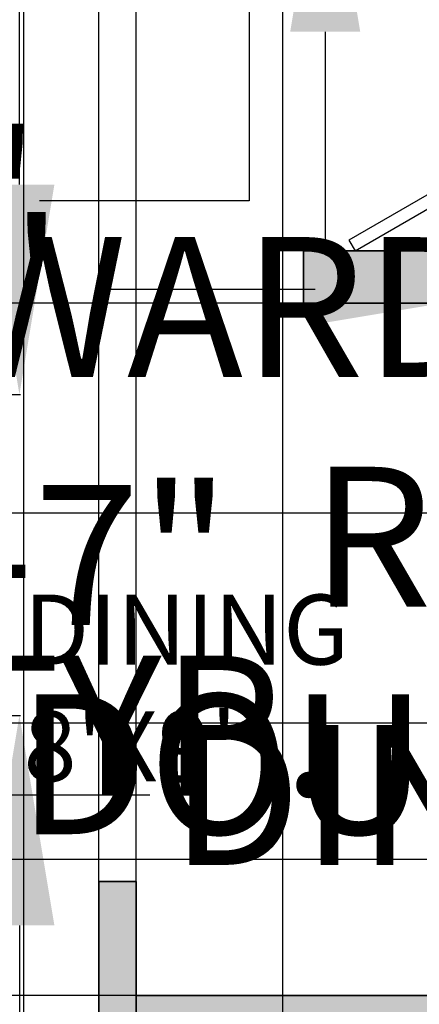
# Model space of a CAD drawing. Units: inches. Extents: x 2838 to 4029, y 1041 to 1915.
# Tile 8 of 16: x 3441 to 3510, y 1377 to 1546. Entities that reach past the tile are written whole.
import ezdxf

# ---------------------------------------------------------------- set-up
doc = ezdxf.new("R2010")
doc.units = ezdxf.units.IN
doc.header["$MEASUREMENT"] = 0
for name, color, linetype, lineweight in [('A-ANNO-DIMS', 2, 'Continuous', 18), ('A-AREA-IDEN', 7, 'Continuous', 18), ('A-DOOR', 3, 'Continuous', 25), ('A-WALL', 7, 'Continuous', 35), ('A-WALL-PATT', 252, 'Continuous', 13)]:
    doc.layers.add(name, color=color, linetype=linetype, lineweight=lineweight)
doc.styles.get("Standard").update_dxf_attribs({"font": 'arial.ttf'})
doc.dimstyles.get("Standard").update_dxf_attribs({"dimtxt": 24, "dimasz": 36, "dimexe": 0.18, "dimexo": 0.0625, "dimgap": 0.09, "dimtad": 0, "dimtih": 1, "dimtoh": 1, "dimdec": 0, "dimzin": 0, "dimdsep": 46, "dimlunit": 3, "dimtxsty": 'Standard', "dimcen": 0.09, "dimadec": 0, "dimazin": 0, "dimtfac": 1, "dimtdec": 0, "dimtofl": 0, "dimtmove": 0, "dimatfit": 3, "dimfxl": 1, "dimtolj": 1, "dimtzin": 0, "dimarcsym": 0})

# ---------------------------------------------------------------- blocks, each defined once
blk = doc.blocks.new('*U3')
for p, q in [((-40, 0), (-40, 6)), ((0, 0), (0, 6))]:
    blk.add_line(p, q)
blk.add_lwpolyline([(0, 0), (-20, -34.64), (-21.52, -33.77), (-1.52, 0.88)], close=True)
blk.add_arc((0, 0), 40, 180, 240)
blk = doc.blocks.new('*D26')
at = {"layer": 'A-ANNO-DIMS', "color": 0, "lineweight": -2, "transparency": 16777216}
for p, q in [((3267.73, 1432.1), (3267.73, 1424.79)), ((3276.73, 1432.1), (3276.73, 1424.79)), ((3231.73, 1424.97), (3195.73, 1424.97)), ((3312.73, 1424.97), (3348.73, 1424.97))]:
    blk.add_line(p, q, dxfattribs=at)
at = {"layer": 'A-ANNO-DIMS', "color": 0, "transparency": 16777216}
for points in [[(3231.73, 1430.97), (3231.73, 1418.97), (3267.73, 1424.97)], [(3312.73, 1430.97), (3312.73, 1418.97), (3276.73, 1424.97)]]:
    blk.add_solid(points, dxfattribs=at)
at = {"layer": 'Defpoints', "color": 0, "transparency": 16777216}
for p in [(3267.73, 1432.17), (3276.73, 1432.17), (3276.73, 1424.97)]:
    blk.add_point(p, dxfattribs=at)
at = {"layer": 'A-ANNO-DIMS', "color": 0, "transparency": 16777216, "insert": (3421.97, 1424.97), "char_height": 24, "attachment_point": 5}
blk.add_mtext('\\A1;0\'-9" TYP.', dxfattribs=at)
blk = doc.blocks.new('*D33')
at = {"layer": 'A-ANNO-DIMS', "color": 0, "lineweight": -2, "transparency": 16777216}
for p, q in [((3601.73, 1469.45), (3601.73, 1505.45)), ((3603.48, 1433.45), (3601.55, 1433.45)), ((3603.48, 1421.37), (3601.55, 1421.37)), ((3601.73, 1385.37), (3601.73, 1349.37)), ((3601.73, 1349.37), (3565.73, 1349.37))]:
    blk.add_line(p, q, dxfattribs=at)
at = {"layer": 'A-ANNO-DIMS', "color": 0, "transparency": 16777216}
for points in [[(3595.73, 1469.45), (3607.73, 1469.45), (3601.73, 1433.45)], [(3595.73, 1385.37), (3607.73, 1385.37), (3601.73, 1421.37)]]:
    blk.add_solid(points, dxfattribs=at)
at = {"layer": 'Defpoints', "color": 0, "transparency": 16777216}
for p in [(3603.54, 1433.45), (3601.73, 1421.37), (3603.54, 1421.37)]:
    blk.add_point(p, dxfattribs=at)
at = {"layer": 'A-ANNO-DIMS', "color": 0, "transparency": 16777216, "insert": (3496.18, 1349.37), "char_height": 24, "attachment_point": 5}
blk.add_mtext('\\A1;TAP 1\'-0"', dxfattribs=at)
blk = doc.blocks.new('*D35')
at = {"layer": 'A-ANNO-DIMS', "color": 0, "lineweight": -2, "transparency": 16777216}
for p, q in [((3480.45, 1632.93), (3480.45, 1668.93)), ((3481.89, 1596.93), (3480.27, 1596.93)), ((3481.89, 1586.93), (3480.27, 1586.93)), ((3480.45, 1550.93), (3480.45, 1514.93)), ((3480.45, 1514.93), (3444.45, 1514.93))]:
    blk.add_line(p, q, dxfattribs=at)
at = {"layer": 'A-ANNO-DIMS', "color": 0, "transparency": 16777216}
for points in [[(3474.45, 1632.93), (3486.45, 1632.93), (3480.45, 1596.93)], [(3474.45, 1550.93), (3486.45, 1550.93), (3480.45, 1586.93)]]:
    blk.add_solid(points, dxfattribs=at)
at = {"layer": 'Defpoints', "color": 0, "transparency": 16777216}
for p in [(3481.95, 1596.93), (3480.45, 1586.93), (3481.95, 1586.93)]:
    blk.add_point(p, dxfattribs=at)
at = {"layer": 'A-ANNO-DIMS', "color": 0, "transparency": 16777216, "insert": (3365.58, 1514.93), "char_height": 24, "attachment_point": 5}
blk.add_mtext('\\A1;TAP 0\'-10"', dxfattribs=at)
blk = doc.blocks.new('*D41')
at = {"layer": 'A-ANNO-DIMS', "color": 0, "lineweight": -2, "transparency": 16777216}
for p, q in [((3284.24, 1506.2), (3284.24, 1496.56)), ((3347.73, 1506.2), (3347.73, 1496.56)), ((3248.24, 1496.74), (3212.24, 1496.74)), ((3383.73, 1496.74), (3419.73, 1496.74))]:
    blk.add_line(p, q, dxfattribs=at)
at = {"layer": 'A-ANNO-DIMS', "color": 0, "transparency": 16777216}
for points in [[(3248.24, 1502.74), (3248.24, 1490.74), (3284.24, 1496.74)], [(3383.73, 1502.74), (3383.73, 1490.74), (3347.73, 1496.74)]]:
    blk.add_solid(points, dxfattribs=at)
at = {"layer": 'Defpoints', "color": 0, "transparency": 16777216}
for p in [(3284.24, 1506.26), (3347.73, 1506.26), (3347.73, 1496.74)]:
    blk.add_point(p, dxfattribs=at)
at = {"layer": 'A-ANNO-DIMS', "color": 0, "transparency": 16777216, "insert": (3624.81, 1496.74), "char_height": 24, "attachment_point": 5}
blk.add_mtext('\\A1;WARDROBE 5\'-3 1/2" TYP.', dxfattribs=at)
blk = doc.blocks.new('*D47')
at = {"layer": 'A-ANNO-DIMS', "color": 0, "lineweight": -2, "transparency": 16777216}
for p, q in [((3493.47, 1640.5), (3493.47, 1676.5)), ((3493.47, 1676.5), (3529.47, 1676.5)), ((3489.85, 1604.5), (3493.65, 1604.5)), ((3489.85, 1579.95), (3493.65, 1579.95)), ((3493.47, 1543.95), (3493.47, 1507.95))]:
    blk.add_line(p, q, dxfattribs=at)
at = {"layer": 'A-ANNO-DIMS', "color": 0, "transparency": 16777216}
for points in [[(3487.47, 1640.5), (3499.47, 1640.5), (3493.47, 1604.5)], [(3487.47, 1543.95), (3499.47, 1543.95), (3493.47, 1579.95)]]:
    blk.add_solid(points, dxfattribs=at)
at = {"layer": 'Defpoints', "color": 0, "transparency": 16777216}
for p in [(3489.78, 1604.5), (3493.47, 1604.5), (3489.78, 1579.95)]:
    blk.add_point(p, dxfattribs=at)
at = {"layer": 'A-ANNO-DIMS', "color": 0, "transparency": 16777216, "insert": (3643.85, 1676.5), "char_height": 24, "attachment_point": 5}
blk.add_mtext('\\A1;BASIN 2\'-0 1/2"', dxfattribs=at)
blk = doc.blocks.new('*D49')
at = {"layer": 'A-ANNO-DIMS', "color": 0, "lineweight": -2, "transparency": 16777216}
for p, q in [((3336.37, 1426.68), (3336.37, 1412.92)), ((3427.37, 1426.68), (3427.37, 1412.92)), ((3372.37, 1413.1), (3391.37, 1413.1)), ((3427.37, 1413.1), (3463.37, 1413.1))]:
    blk.add_line(p, q, dxfattribs=at)
at = {"layer": 'A-ANNO-DIMS', "color": 0, "transparency": 16777216}
for points in [[(3372.37, 1419.1), (3372.37, 1407.1), (3336.37, 1413.1)], [(3391.37, 1419.1), (3391.37, 1407.1), (3427.37, 1413.1)]]:
    blk.add_solid(points, dxfattribs=at)
at = {"layer": 'Defpoints', "color": 0, "transparency": 16777216}
for p in [(3336.37, 1426.75), (3427.37, 1426.75), (3427.37, 1413.1)]:
    blk.add_point(p, dxfattribs=at)
at = {"layer": 'A-ANNO-DIMS', "color": 0, "transparency": 16777216, "insert": (3595.36, 1413.1), "char_height": 24, "attachment_point": 5}
blk.add_mtext('\\A1;DINING SET 7\'-7"', dxfattribs=at)
blk = doc.blocks.new('*D50')
at = {"layer": 'A-ANNO-DIMS', "color": 0, "lineweight": -2, "transparency": 16777216}
for p, q in [((3441.02, 1517.75), (3441.02, 1553.75)), ((3427.44, 1481.75), (3441.2, 1481.75)), ((3427.44, 1426.75), (3441.2, 1426.75)), ((3441.02, 1390.75), (3441.02, 1354.75))]:
    blk.add_line(p, q, dxfattribs=at)
at = {"layer": 'A-ANNO-DIMS', "color": 0, "transparency": 16777216}
for points in [[(3435.02, 1517.75), (3447.02, 1517.75), (3441.02, 1481.75)], [(3435.02, 1390.75), (3447.02, 1390.75), (3441.02, 1426.75)]]:
    blk.add_solid(points, dxfattribs=at)
at = {"layer": 'Defpoints', "color": 0, "transparency": 16777216}
for p in [(3427.37, 1481.75), (3441.02, 1481.75), (3427.37, 1426.75)]:
    blk.add_point(p, dxfattribs=at)
at = {"layer": 'A-ANNO-DIMS', "color": 0, "transparency": 16777216, "insert": (3441.02, 1454.25), "char_height": 24, "attachment_point": 5}
blk.add_mtext('\\A1;4\'-7"', dxfattribs=at)
blk = doc.blocks.new('*D53')
at = {"layer": 'A-ANNO-DIMS', "color": 0, "lineweight": -2, "transparency": 16777216}
for p, q in [((3583.96, 1508.36), (3583.96, 1544.36)), ((3588.4, 1472.36), (3583.78, 1472.36)), ((3588.4, 1442.36), (3583.78, 1442.36)), ((3583.96, 1406.36), (3583.96, 1370.36))]:
    blk.add_line(p, q, dxfattribs=at)
at = {"layer": 'A-ANNO-DIMS', "color": 0, "transparency": 16777216}
for points in [[(3577.96, 1508.36), (3589.96, 1508.36), (3583.96, 1472.36)], [(3577.96, 1406.36), (3589.96, 1406.36), (3583.96, 1442.36)]]:
    blk.add_solid(points, dxfattribs=at)
at = {"layer": 'Defpoints', "color": 0, "transparency": 16777216}
for p in [(3588.46, 1472.36), (3583.96, 1442.36), (3588.46, 1442.36)]:
    blk.add_point(p, dxfattribs=at)
at = {"layer": 'A-ANNO-DIMS', "color": 0, "transparency": 16777216, "insert": (3583.96, 1457.36), "char_height": 24, "attachment_point": 5}
blk.add_mtext('\\A1;RANGE 2\'-6"', dxfattribs=at)
blk = doc.blocks.new('*D55')
at = {"layer": 'A-ANNO-DIMS', "color": 0, "lineweight": -2, "transparency": 16777216}
for p, q in [((3491.76, 1499.78), (3455.76, 1499.78)), ((3527.76, 1494.67), (3527.76, 1499.96)), ((3562.26, 1494.67), (3562.26, 1499.96)), ((3598.26, 1499.78), (3634.26, 1499.78))]:
    blk.add_line(p, q, dxfattribs=at)
at = {"layer": 'A-ANNO-DIMS', "color": 0, "transparency": 16777216}
for points in [[(3491.76, 1505.78), (3491.76, 1493.78), (3527.76, 1499.78)], [(3598.26, 1505.78), (3598.26, 1493.78), (3562.26, 1499.78)]]:
    blk.add_solid(points, dxfattribs=at)
at = {"layer": 'Defpoints', "color": 0, "transparency": 16777216}
for p in [(3527.76, 1499.78), (3527.76, 1494.6), (3562.26, 1494.6)]:
    blk.add_point(p, dxfattribs=at)
at = {"layer": 'A-ANNO-DIMS', "color": 0, "transparency": 16777216, "insert": (3260.33, 1499.78), "char_height": 24, "attachment_point": 5}
blk.add_mtext('\\A1;BASE CABINET 2\'-10 1/2"', dxfattribs=at)
blk = doc.blocks.new('*D57')
at = {"layer": 'A-ANNO-DIMS', "color": 0, "lineweight": -2, "transparency": 16777216}
for p, q in [((3585.57, 1472.38), (3585.57, 1508.38)), ((3590.9, 1436.38), (3585.39, 1436.38)), ((3590.9, 1400.38), (3585.39, 1400.38)), ((3585.57, 1364.38), (3585.57, 1328.38))]:
    blk.add_line(p, q, dxfattribs=at)
at = {"layer": 'A-ANNO-DIMS', "color": 0, "transparency": 16777216}
for points in [[(3579.57, 1472.38), (3591.57, 1472.38), (3585.57, 1436.38)], [(3579.57, 1364.38), (3591.57, 1364.38), (3585.57, 1400.38)]]:
    blk.add_solid(points, dxfattribs=at)
at = {"layer": 'Defpoints', "color": 0, "transparency": 16777216}
for p in [(3590.97, 1436.38), (3585.57, 1400.38), (3590.97, 1400.38)]:
    blk.add_point(p, dxfattribs=at)
at = {"layer": 'A-ANNO-DIMS', "color": 0, "transparency": 16777216, "insert": (3585.57, 1418.38), "char_height": 24, "attachment_point": 5}
blk.add_mtext('\\A1;DOUBLE SINK 3\'-0"', dxfattribs=at)
blk = doc.blocks.new('*D73')
at = {"layer": 'A-ANNO-DIMS', "color": 0, "lineweight": -2, "transparency": 16777216}
for p, q in [((3461.038746, 1200.359846), (3461.038746, 1711.702346)), ((3618.731626, 1200.359846), (3618.731626, 1711.702346)), ((3425.038746, 1711.522346), (3389.038746, 1711.522346)), ((3654.731626, 1711.522346), (3690.731626, 1711.522346))]:
    blk.add_line(p, q, dxfattribs=at)
at = {"layer": 'A-ANNO-DIMS', "color": 0, "transparency": 16777216}
for points in [[(3425.038746, 1717.522346), (3425.038746, 1705.522346), (3461.038746, 1711.522346)], [(3654.731626, 1717.522346), (3654.731626, 1705.522346), (3618.731626, 1711.522346)]]:
    blk.add_solid(points, dxfattribs=at)
at = {"layer": 'Defpoints', "color": 0, "transparency": 16777216}
for p in [(3618.731626, 1711.522346), (3461.038746, 1200.297346), (3618.731626, 1200.297346)]:
    blk.add_point(p, dxfattribs=at)
at = {"layer": 'A-ANNO-DIMS', "color": 0, "transparency": 16777216, "insert": (3539.885186, 1711.522346), "char_height": 24, "attachment_point": 5}
blk.add_mtext('\\A1;13\'-1 1/2"', dxfattribs=at)
blk = doc.blocks.new('*D78')
at = {"layer": 'A-ANNO-DIMS', "color": 0, "lineweight": -2, "transparency": 16777216}
for p, q in [((3667.956626, 1590.394218), (3667.956626, 1626.394218)), ((3498.794126, 1554.394218), (3668.136626, 1554.394218)), ((3498.638013, 1506.394218), (3668.136626, 1506.394218)), ((3667.956626, 1470.394218), (3667.956626, 1434.394218))]:
    blk.add_line(p, q, dxfattribs=at)
at = {"layer": 'A-ANNO-DIMS', "color": 0, "transparency": 16777216}
for points in [[(3661.956626, 1590.394218), (3673.956626, 1590.394218), (3667.956626, 1554.394218)], [(3661.956626, 1470.394218), (3673.956626, 1470.394218), (3667.956626, 1506.394218)]]:
    blk.add_solid(points, dxfattribs=at)
at = {"layer": 'Defpoints', "color": 0, "transparency": 16777216}
for p in [(3498.731626, 1554.394218), (3667.956626, 1554.394218), (3498.575513, 1506.394218)]:
    blk.add_point(p, dxfattribs=at)
at = {"layer": 'A-ANNO-DIMS', "color": 0, "transparency": 16777216, "insert": (3667.956626, 1530.394218), "char_height": 24, "attachment_point": 5}
blk.add_mtext('\\A1;4\'-0"', dxfattribs=at)
blk = doc.blocks.new('*D79')
at = {"layer": 'A-ANNO-DIMS', "color": 0, "lineweight": -2, "transparency": 16777216}
for p, q in [((3379.05, 1400.64), (3379.05, 1711.7)), ((3454.63, 1398.31), (3454.63, 1711.7)), ((3415.05, 1711.52), (3418.63, 1711.52)), ((3454.63, 1711.52), (3490.63, 1711.52))]:
    blk.add_line(p, q, dxfattribs=at)
at = {"layer": 'A-ANNO-DIMS', "color": 0, "transparency": 16777216}
for points in [[(3415.05, 1717.52), (3415.05, 1705.52), (3379.05, 1711.52)], [(3418.63, 1717.52), (3418.63, 1705.52), (3454.63, 1711.52)]]:
    blk.add_solid(points, dxfattribs=at)
at = {"layer": 'Defpoints', "color": 0, "transparency": 16777216}
for p in [(3454.63, 1711.52), (3379.05, 1400.57), (3454.63, 1398.25)]:
    blk.add_point(p, dxfattribs=at)
at = {"layer": 'A-ANNO-DIMS', "color": 0, "transparency": 16777216, "insert": (3550.65, 1711.52), "char_height": 24, "attachment_point": 5}
blk.add_mtext('\\A1;6\'-3 1/2"', dxfattribs=at)
blk = doc.blocks.new('*D82')
at = {"layer": 'A-ANNO-DIMS', "color": 0, "lineweight": -2, "transparency": 16777216}
for p, q in [((3405.73, 1573.06), (3405.73, 1081.89)), ((3441.73, 1569.23), (3441.73, 1081.89)), ((3369.73, 1082.07), (3333.73, 1082.07)), ((3477.73, 1082.07), (3513.73, 1082.07))]:
    blk.add_line(p, q, dxfattribs=at)
at = {"layer": 'A-ANNO-DIMS', "color": 0, "transparency": 16777216}
for points in [[(3369.73, 1088.07), (3369.73, 1076.07), (3405.73, 1082.07)], [(3477.73, 1088.07), (3477.73, 1076.07), (3441.73, 1082.07)]]:
    blk.add_solid(points, dxfattribs=at)
at = {"layer": 'Defpoints', "color": 0, "transparency": 16777216}
for p in [(3405.73, 1573.12), (3441.73, 1569.3), (3441.73, 1082.07)]:
    blk.add_point(p, dxfattribs=at)
at = {"layer": 'A-ANNO-DIMS', "color": 0, "transparency": 16777216, "insert": (3545.71, 1082.07), "char_height": 24, "attachment_point": 5}
blk.add_mtext('\\A1;3\'-0"', dxfattribs=at)
blk = doc.blocks.new('*D87')
at = {"layer": 'A-ANNO-DIMS', "color": 0, "lineweight": -2, "transparency": 16777216}
for p, q in [((3227.506626, 1497.394218), (3227.506626, 1533.394218)), ((3513.669126, 1461.394218), (3227.326626, 1461.394218)), ((3513.669126, 1425.394218), (3227.326626, 1425.394218)), ((3227.506626, 1389.394218), (3227.506626, 1353.394218))]:
    blk.add_line(p, q, dxfattribs=at)
at = {"layer": 'A-ANNO-DIMS', "color": 0, "transparency": 16777216}
for points in [[(3221.506626, 1497.394218), (3233.506626, 1497.394218), (3227.506626, 1461.394218)], [(3221.506626, 1389.394218), (3233.506626, 1389.394218), (3227.506626, 1425.394218)]]:
    blk.add_solid(points, dxfattribs=at)
at = {"layer": 'Defpoints', "color": 0, "transparency": 16777216}
for p in [(3227.506626, 1461.394218), (3513.731626, 1461.394218), (3513.731626, 1425.394218)]:
    blk.add_point(p, dxfattribs=at)
at = {"layer": 'A-ANNO-DIMS', "color": 0, "transparency": 16777216, "insert": (3227.506626, 1443.394218), "char_height": 24, "attachment_point": 5}
blk.add_mtext('\\A1;3\'-0"', dxfattribs=at)
blk = doc.blocks.new('*D91')
at = {"layer": 'A-ANNO-DIMS', "color": 0, "lineweight": -2, "transparency": 16777216}
for p, q in [((3227.506626, 1533.394218), (3227.506626, 1569.394218)), ((3522.669126, 1497.394218), (3227.326626, 1497.394218)), ((3522.669126, 1461.394218), (3227.326626, 1461.394218)), ((3227.506626, 1425.394218), (3227.506626, 1389.394218))]:
    blk.add_line(p, q, dxfattribs=at)
at = {"layer": 'A-ANNO-DIMS', "color": 0, "transparency": 16777216}
for points in [[(3221.506626, 1533.394218), (3233.506626, 1533.394218), (3227.506626, 1497.394218)], [(3221.506626, 1425.394218), (3233.506626, 1425.394218), (3227.506626, 1461.394218)]]:
    blk.add_solid(points, dxfattribs=at)
at = {"layer": 'Defpoints', "color": 0, "transparency": 16777216}
for p in [(3522.731626, 1497.394218), (3227.506626, 1461.394218), (3522.731626, 1461.394218)]:
    blk.add_point(p, dxfattribs=at)
at = {"layer": 'A-ANNO-DIMS', "color": 0, "transparency": 16777216, "insert": (3227.506626, 1479.394218), "char_height": 24, "attachment_point": 5}
blk.add_mtext('\\A1;3\'-0"', dxfattribs=at)
blk = doc.blocks.new('*D93')
at = {"layer": 'A-ANNO-DIMS', "color": 0, "lineweight": -2, "transparency": 16777216}
for p, q in [((3227.51, 1438.06), (3227.51, 1474.06)), ((3227.51, 1474.06), (3263.51, 1474.06)), ((3522.67, 1402.06), (3227.33, 1402.06)), ((3522.67, 1378.73), (3227.33, 1378.73)), ((3227.51, 1342.73), (3227.51, 1306.73))]:
    blk.add_line(p, q, dxfattribs=at)
at = {"layer": 'A-ANNO-DIMS', "color": 0, "transparency": 16777216}
for points in [[(3221.51, 1438.06), (3233.51, 1438.06), (3227.51, 1402.06)], [(3221.51, 1342.73), (3233.51, 1342.73), (3227.51, 1378.73)]]:
    blk.add_solid(points, dxfattribs=at)
at = {"layer": 'Defpoints', "color": 0, "transparency": 16777216}
for p in [(3227.51, 1402.06), (3522.73, 1402.06), (3522.73, 1378.73)]:
    blk.add_point(p, dxfattribs=at)
at = {"layer": 'A-ANNO-DIMS', "color": 0, "transparency": 16777216, "insert": (3331.65, 1474.06), "char_height": 24, "attachment_point": 5}
blk.add_mtext('\\A1;1\'-11 1/2"', dxfattribs=at)
blk = doc.blocks.new('*D101')
at = {"layer": 'A-ANNO-DIMS', "color": 0, "lineweight": -2, "transparency": 16777216}
for p, q in [((3461.04, 1200.36), (3461.04, 1711.7)), ((3486.18, 1200.36), (3486.18, 1711.7)), ((3425.04, 1711.52), (3389.04, 1711.52)), ((3522.18, 1711.52), (3558.18, 1711.52))]:
    blk.add_line(p, q, dxfattribs=at)
at = {"layer": 'A-ANNO-DIMS', "color": 0, "transparency": 16777216}
for points in [[(3425.04, 1717.52), (3425.04, 1705.52), (3461.04, 1711.52)], [(3522.18, 1717.52), (3522.18, 1705.52), (3486.18, 1711.52)]]:
    blk.add_solid(points, dxfattribs=at)
at = {"layer": 'Defpoints', "color": 0, "transparency": 16777216}
for p in [(3486.18, 1711.52), (3461.04, 1200.3), (3486.18, 1200.3)]:
    blk.add_point(p, dxfattribs=at)
at = {"layer": 'A-ANNO-DIMS', "color": 0, "transparency": 16777216, "insert": (3590.37, 1711.52), "char_height": 24, "attachment_point": 5}
blk.add_mtext('\\A1;2\'-1"', dxfattribs=at)
blk = doc.blocks.new('*D103')
at = {"layer": 'A-ANNO-DIMS', "color": 0, "lineweight": -2, "transparency": 16777216}
for p, q in [((3227.51, 1628.55), (3227.51, 1664.55)), ((3227.51, 1664.55), (3263.51, 1664.55)), ((3469.64, 1592.55), (3227.33, 1592.55)), ((3441.67, 1578.3), (3227.33, 1578.3)), ((3227.51, 1542.3), (3227.51, 1506.3))]:
    blk.add_line(p, q, dxfattribs=at)
at = {"layer": 'A-ANNO-DIMS', "color": 0, "transparency": 16777216}
for points in [[(3221.51, 1628.55), (3233.51, 1628.55), (3227.51, 1592.55)], [(3221.51, 1542.3), (3233.51, 1542.3), (3227.51, 1578.3)]]:
    blk.add_solid(points, dxfattribs=at)
at = {"layer": 'Defpoints', "color": 0, "transparency": 16777216}
for p in [(3227.51, 1592.55), (3469.7, 1592.55), (3441.73, 1578.3)]:
    blk.add_point(p, dxfattribs=at)
at = {"layer": 'A-ANNO-DIMS', "color": 0, "transparency": 16777216, "insert": (3322.33, 1664.55), "char_height": 24, "attachment_point": 5}
blk.add_mtext('\\A1;1\'-2 1/2"', dxfattribs=at)

msp = doc.modelspace()

# ---------------------------------------------------------------- hatches: boundary and pattern name
at = {"layer": 'A-WALL-PATT'}
h = msp.add_hatch(color=256, dxfattribs=at)
h.dxf.hatch_style = 1
h.paths.add_polyline_path([(3427.52, 1671.3), (3360.91, 1671.3), (3360.91, 1662.3), (3396.73, 1662.3), (3396.73, 1554.39), (3397.12, 1554.39, -0.007312), (3398.53, 1554.41), (3405.73, 1554.41), (3405.73, 1662.3), (3427.52, 1662.3)])
h.paths.add_polyline_path([(3546.42, 1671.3), (3451.52, 1671.3), (3451.52, 1662.3), (3489.73, 1662.3), (3489.73, 1592.86, -0.016107), (3489.73, 1591.9), (3489.73, 1578.3), (3441.73, 1578.3), (3441.73, 1569.3), (3489.73, 1569.3), (3489.73, 1554.41), (3498.73, 1554.41), (3498.73, 1662.3), (3546.42, 1662.3)])
h.paths.add_polyline_path([(3627.73, 1671.3), (3594.42, 1671.3), (3594.42, 1662.3), (3618.73, 1662.3), (3618.73, 1634.03), (3627.73, 1634.03)])
h.paths.add_polyline_path([(3627.73, 1586.03), (3618.73, 1586.03), (3618.73, 1506.39), (3545.12, 1506.39), (3489.73, 1506.39), (3489.73, 1497.39), (3513.73, 1497.39), (3618.73, 1497.39), (3618.73, 1469.85), (3627.73, 1469.85)])
h.paths.add_polyline_path([(3627.73, 1421.85), (3618.73, 1421.85), (3618.73, 1378.73), (3522.73, 1378.73), (3513.73, 1378.73), (3461.04, 1378.73), (3461.04, 1369.73), (3513.73, 1369.73), (3618.73, 1369.73), (3618.73, 1320.94), (3627.73, 1320.94)])
h.paths.add_polyline_path([(3627.73, 1272.94), (3618.73, 1272.94), (3618.73, 1200.3), (3599.07, 1200.3), (3599.07, 1191.3), (3627.73, 1191.3)])
h.paths.add_polyline_path([(3551.07, 1200.3), (3510.18, 1200.3), (3510.18, 1191.3), (3551.07, 1191.3)])
h.paths.add_polyline_path([(3486.18, 1200.3), (3461.04, 1200.3), (3461.04, 1398.25), (3454.63, 1398.25), (3454.63, 1200.3), (3432.45, 1200.3), (3432.45, 1191.3), (3486.18, 1191.3)])
h.paths.add_polyline_path([(3300.73, 1200.3), (3276.73, 1200.3), (3276.73, 1391.57), (3331.05, 1391.57), (3331.05, 1400.57), (3276.73, 1400.57), (3276.73, 1432.17), (3267.73, 1432.17), (3267.73, 1191.3), (3300.73, 1191.3)])

# ---------------------------------------------------------------- linework, layer by layer
at = {"layer": 'A-WALL'}
for p, q in [((3618.73, 1506.39), (3489.73, 1506.39)), ((3489.73, 1506.39), (3489.73, 1497.39)), ((3618.73, 1506.39), (3489.73, 1506.39)), ((3489.73, 1506.39), (3489.73, 1497.39)), ((3491.37, 1506.39), (3618.73, 1506.39)), ((3618.73, 1497.39), (3489.73, 1497.39)), ((3489.73, 1497.39), (3513.73, 1497.39)), ((3454.63, 1200.3), (3454.63, 1398.25)), ((3461.04, 1398.25), (3454.63, 1398.25)), ((3461.04, 1398.25), (3454.63, 1398.25)), ((3454.63, 1398.25), (3454.63, 1200.3)), ((3461.04, 1200.3), (3461.04, 1398.25)), ((3461.04, 1378.73), (3461.04, 1398.25)), ((3513.73, 1378.73), (3461.04, 1378.73)), ((3513.73, 1378.73), (3461.04, 1378.73))]:
    msp.add_line(p, q, dxfattribs=at)

# ---------------------------------------------------------------- block references
at = {"layer": 'A-DOOR', "xscale": -1.200513446172712, "yscale": 1.200513446172712, "zscale": 1.200513446172712, "rotation": 90}
msp.add_blockref('*U3', (3498.58, 1506.39), dxfattribs=at)

# ---------------------------------------------------------------- texts
at = {"layer": 'A-AREA-IDEN', "insert": (3441.73, 1447.45), "char_height": 12, "attachment_point": 1}
msp.add_mtext_dynamic_manual_height_columns("DINING\\P8'X9'", width=64.6015, gutter_width=1, heights=[0], dxfattribs=at)

# ---------------------------------------------------------------- dimensions: what is measured, and where the dimension line sits
at = {"layer": 'A-ANNO-DIMS'}
for base, p1, p2, picture, middle in [((3454.63, 1711.52), (3379.05, 1400.57), (3454.63, 1398.25), '*D79', (3550.65, 1711.52)), ((3618.73, 1711.52), (3461.04, 1200.3), (3618.73, 1200.3), '*D73', (3539.89, 1711.52)), ((3486.18, 1711.52), (3461.04, 1200.3), (3486.18, 1200.3), '*D101', (3590.37, 1711.52)), ((3441.73, 1082.07), (3405.73, 1573.12), (3441.73, 1569.3), '*D82', (3545.71, 1082.07))]:
    dim = msp.add_linear_dim(base=base, p1=p1, p2=p2, dimstyle='Standard', override={"dimdec": 1, "dimlfac": 1, "dimrnd": 0, "dimzin": 1, "dimdsep": 46, "dimlunit": 4, "dimfrac": 2}, dxfattribs=at)
    dim.commit()
    dim.dimension.update_dxf_attribs({"geometry": picture, "text_midpoint": middle})
for base, p1, p2, angle, text, picture, middle in [((3493.4667, 1604.5013), (3489.7841, 1579.9504), (3489.7841, 1604.5013), 90, 'BASIN <>', '*D47', (3643.8514, 1676.5013)), ((3480.45, 1586.93), (3481.95, 1596.93), (3481.95, 1586.93), 270, 'TAP <>', '*D35', (3365.58, 1514.93)), ((3527.76, 1499.78), (3562.26, 1494.6), (3527.76, 1494.6), 180, 'BASE CABINET <>', '*D55', (3260.33, 1499.78)), ((3583.96, 1442.36), (3588.46, 1472.36), (3588.46, 1442.36), 270, 'RANGE <>', '*D53', (3583.96, 1457.36)), ((3585.57, 1400.38), (3590.97, 1436.38), (3590.97, 1400.38), 270, 'DOUBLE SINK <>', '*D57', (3585.57, 1418.38)), ((3601.73, 1421.37), (3603.54, 1433.45), (3603.54, 1421.37), 270, 'TAP <>', '*D33', (3496.18, 1349.37))]:
    dim = msp.add_linear_dim(base=base, p1=p1, p2=p2, angle=angle, text=text, dimstyle='Standard', override={"dimdec": 1, "dimlfac": 1, "dimrnd": 0, "dimzin": 1, "dimdsep": 46, "dimlunit": 4, "dimfrac": 2}, dxfattribs=at)
    dim.commit()
    dim.dimension.update_dxf_attribs({"geometry": picture, "text_midpoint": middle})
for base, p1, p2, picture, middle in [((3227.5066, 1592.5486), (3441.7316, 1578.2973), (3469.6999, 1592.5486), '*D103', (3322.3279, 1664.5486)), ((3667.96, 1554.39), (3498.58, 1506.39), (3498.73, 1554.39), '*D78', (3667.96, 1530.39)), ((3227.51, 1461.39), (3522.73, 1497.39), (3522.73, 1461.39), '*D91', (3227.51, 1479.39)), ((3441.02, 1481.75), (3427.37, 1426.75), (3427.37, 1481.75), '*D50', (3441.02, 1454.25)), ((3227.51, 1461.39), (3513.73, 1425.39), (3513.73, 1461.39), '*D87', (3227.51, 1443.39)), ((3227.51, 1402.06), (3522.73, 1378.73), (3522.73, 1402.06), '*D93', (3331.65, 1474.06))]:
    dim = msp.add_linear_dim(base=base, p1=p1, p2=p2, angle=90, dimstyle='Standard', override={"dimdec": 1, "dimlfac": 1, "dimrnd": 0, "dimzin": 1, "dimdsep": 46, "dimlunit": 4, "dimfrac": 2}, dxfattribs=at)
    dim.commit()
    dim.dimension.update_dxf_attribs({"geometry": picture, "text_midpoint": middle})
for base, p1, p2, text, picture, middle in [((3347.73, 1496.74), (3284.24, 1506.26), (3347.73, 1506.26), 'WARDROBE <> TYP.', '*D41', (3624.81, 1496.74)), ((3427.37, 1413.1), (3336.37, 1426.75), (3427.37, 1426.75), 'DINING SET <>', '*D49', (3595.36, 1413.1)), ((3276.73, 1424.97), (3267.73, 1432.17), (3276.73, 1432.17), '<> TYP.', '*D26', (3421.97, 1424.97))]:
    dim = msp.add_linear_dim(base=base, p1=p1, p2=p2, text=text, dimstyle='Standard', override={"dimdec": 1, "dimlfac": 1, "dimrnd": 0, "dimzin": 1, "dimdsep": 46, "dimlunit": 4, "dimfrac": 2}, dxfattribs=at)
    dim.commit()
    dim.dimension.update_dxf_attribs({"geometry": picture, "text_midpoint": middle})

doc.saveas('drawing.dxf')
